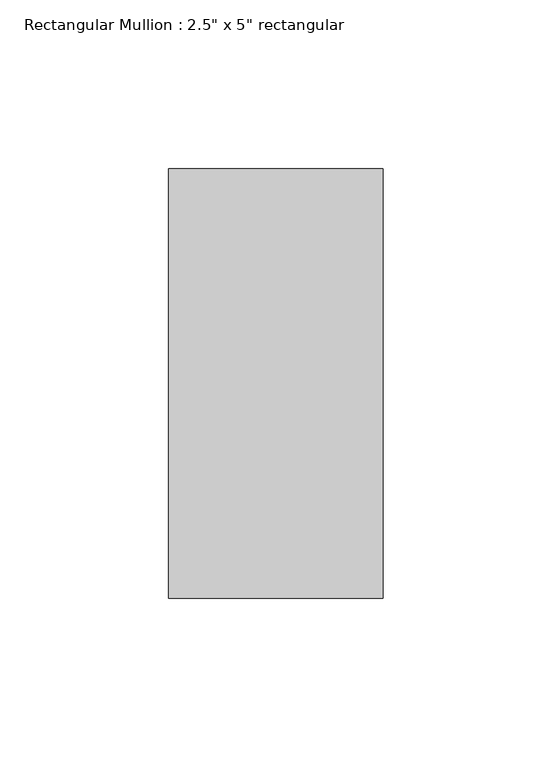
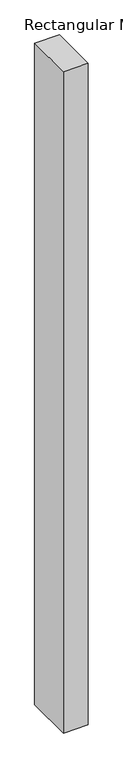
"""IFC4 building model written with IfcOpenShell, lengths in millimetres: member geometry."""

from ifc_helpers import new_model, si_unit, frame, origin, place, context, project, spatial, polyline, outline, extrude, source, transform, mapped, element, save


def member_18831802(model_context):
    return source(origin(), model_context, "Body", "SweptSolid", [
        extrude(outline(polyline([(31.75, 63.5), (31.75, -63.5), (-31.75, -63.5), (-31.75, 63.5), (31.75, 63.5)])), frame((0.0, 0.0, -1789.0304763), z_axis=(0.0, 0.0, 1.0), x_axis=(1.0, 0.0, 0.0)), (0.0, 0.0, 1.0), 1789.0304763),
    ])


if __name__ == "__main__":
    model = new_model("IFC4")
    model_context = context("Model", 3, world=origin())
    ifc_project = project(units=[si_unit("LENGTHUNIT", "METRE", prefix="MILLI")], contexts=[model_context])
    site = spatial("IfcSite", under=ifc_project)
    building = spatial("IfcBuilding", under=site)
    placement = place(None, origin())
    member_shape = member_18831802(model_context)
    element("IfcMember", 1, ObjectType="Rectangular Mullion : 2.5\" x 5\" rectangular", at=placement, inside=building, context=model_context, shape_type="MappedRepresentation", body=[
        mapped(member_shape, transform((0.0, 0.0, 0.0), x_axis=(1.0, 0.0, 0.0), y_axis=(0.0, 1.0, 0.0), z_axis=(0.0, 0.0, 1.0))),
    ])
    save(model, "model.ifc")

# Revit data of these elements
# Type "Rectangular Mullion : 2.5\" x 5\" rectangular"
#   built-in parameter 1007304 = 0.416667 (stored number, unit not read)
#   built-in parameter 1007301 = 0.104167 (stored number, unit not read)
#   built-in parameter 1007300 = 0.104167 (stored number, unit not read)
# Element 1 (IfcMember, "Rectangular Mullion : 2.5\" x 5\" rectangular")
#   Materials on its faces: "Aluminum"
# Materials
#   "Aluminum": class "Metal", colour RGB 247 247 247, transparency 0, Description = "Aluminum 6061", Cost = 0
